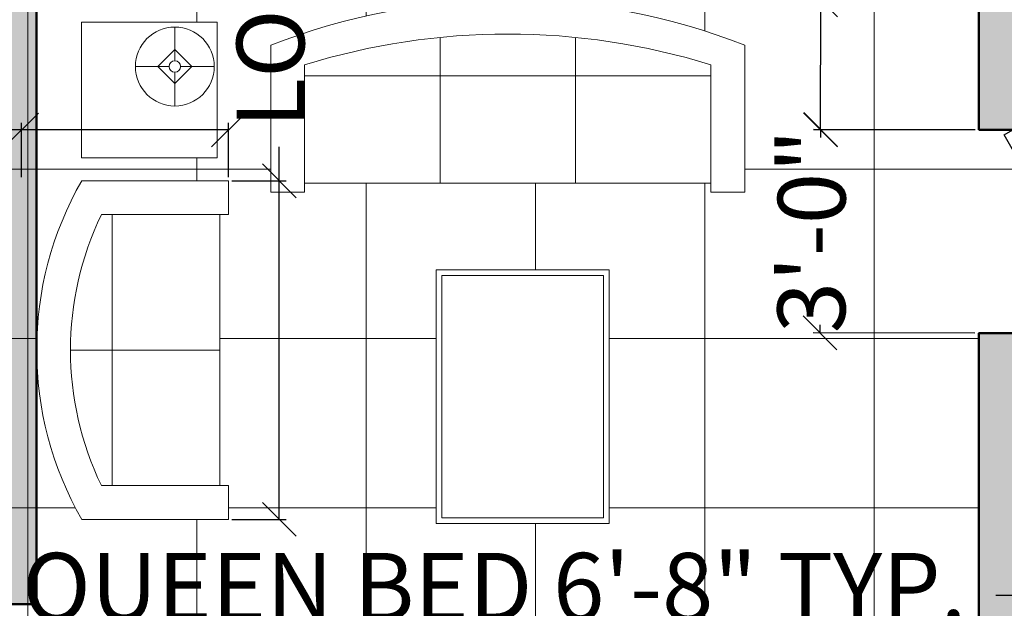
# Model space of a CAD drawing. Units: inches. Extents: x 2371 to 3019, y 129 to 700.
# Tile 8 of 14: x 2579 to 2753, y 432 to 537. Entities that reach past the tile are written whole.
import ezdxf

# ---------------------------------------------------------------- set-up
doc = ezdxf.new("R2010")
doc.units = ezdxf.units.IN
for name, color, linetype, lineweight in [('A-ANNO-DIMS', 2, 'Continuous', 18), ('A-DOOR', 4, 'Continuous', 25), ('A-FLOR-PATT', 252, 'Continuous', 13), ('A-FURN', 8, 'Continuous', 18), ('A-WALL', 7, 'Continuous', 50), ('A-WALL-PATT', 8, 'Continuous', 13)]:
    doc.layers.add(name, color=color, linetype=linetype, lineweight=lineweight)
doc.styles.get("Standard").update_dxf_attribs({"font": 'arial.ttf'})
doc.dimstyles.new('ISO-25', dxfattribs={"dimtxt": 12, "dimasz": 6, "dimexe": 1.25, "dimexo": 0.625, "dimtad": 0, "dimdec": 1, "dimlunit": 3, "dimtxsty": 'Standard', "dimblk": 'OBLIQUE', "dimblk1": 'ORIGIN2', "dimblk2": 'OBLIQUE', "dimcen": 2.5, "dimadec": 0, "dimazin": 0, "dimtfac": 1, "dimtdec": 1, "dimtmove": 0, "dimatfit": 3, "dimldrblk": 'OBLIQUE', "dimfxl": 1, "dimarcsym": 0})

# ---------------------------------------------------------------- blocks, each defined once
blk = doc.blocks.new('Sofa - Roundback Loveseat 5 ft.')
for p, q in [((0, -32.44198), (0, -5.99998)), ((-24, -33.99998), (-24, -11.46958)), ((24.00004, -33.99998), (24.00004, -11.46958)), ((-23.9998, -13.38178), (23.99986, -13.38178)), ((-24, -32.44198), (24.00004, -32.44198))]:
    blk.add_line(p, q)
for points in [[(-24, -33.99998), (-30, -33.99998), (-30, -7.99998)], [(30.00004, -7.99998), (30.00004, -33.99998), (24.00004, -33.99998)]]:
    blk.add_lwpolyline(points)
for centre, radius, start, end in [((0, -60.24998), 60.24998, 60.13715, 119.8628), ((0, -61.38438), 55.38444, 64.32083, 115.6792)]:
    blk.add_arc(centre, radius, start, end)
blk = doc.blocks.new('Sofa - Roundback 7 ft.')
for p, q in [((-12.00002, -32.4421), (-12.00003, -6.5971)), ((11.99997, -32.4421), (11.99998, -6.5971)), ((-36.000027, -34), (-36.000027, -11.4696)), ((35.99998, -34), (35.99998, -11.4696)), ((-35.999844, -13.3819), (35.9998, -13.3819)), ((-36.000027, -32.4421), (35.99998, -32.4421))]:
    blk.add_line(p, q)
for points in [[(-36.000027, -34), (-42.000027, -34), (-42.000027, -8)], [(41.99998, -8), (41.99998, -34), (35.99998, -34)]]:
    blk.add_lwpolyline(points)
for centre, radius, start, end in [((0, -114.25), 114.25, 68.43141, 111.5686), ((-0.00001, -127.1968), 121.1968, 72.72033, 107.2797)]:
    blk.add_arc(centre, radius, start, end)
blk = doc.blocks.new('Lamp - Table')
for p, q in [((0, 7), (0, 1)), ((0, 3), (-3, 0)), ((3, 0), (0, 3)), ((-1, 0), (-7, 0)), ((-3, 0), (0, -3)), ((0, -3), (3, 0)), ((1, 0), (7, 0)), ((0, -1), (0, -7))]:
    blk.add_line(p, q)
for radius in [7, 1]:
    blk.add_circle((0, 0), radius)
blk = doc.blocks.new('*U10')
for p, q in [((0, 0), (0, -6)), ((36, 0), (36, -6))]:
    blk.add_line(p, q)
blk.add_lwpolyline([(0, 0), (31.18, 18), (32.05, 16.48), (0.87, -1.52)], close=True)
blk.add_arc((0, 0), 36, 0, 30)
blk = doc.blocks.new('_Oblique')
at = {"color": 0, "linetype": 'ByBlock', "lineweight": -2}
blk.add_line((-0.5, -0.5), (0.5, 0.5), dxfattribs=at)
blk = doc.blocks.new('*D24')
at = {"layer": 'A-ANNO-DIMS', "color": 0, "lineweight": -2, "transparency": 16777216}
for p, q in [((2757.61, 423.1), (2757.61, 435.73)), ((2837.61, 423.1), (2837.61, 435.73)), ((2757.61, 434.48), (2751.61, 434.48)), ((2837.61, 434.48), (2757.61, 434.48))]:
    blk.add_line(p, q, dxfattribs=at)
at = {"layer": 'Defpoints', "color": 0, "lineweight": 25, "transparency": 16777216}
for p in [(2757.61, 434.48), (2757.61, 422.48), (2837.61, 422.48)]:
    blk.add_point(p, dxfattribs=at)
at = {"layer": 'A-ANNO-DIMS', "color": 0, "lineweight": -2, "transparency": 16777216, "xscale": 6, "yscale": 6, "zscale": 6, "rotation": 180}
blk.add_blockref('_Oblique', (2757.61, 434.48), dxfattribs=at)
at = {"layer": 'A-ANNO-DIMS', "color": 0, "lineweight": -2, "transparency": 16777216, "xscale": 6, "yscale": 6, "zscale": 6}
blk.add_blockref('_Oblique', (2837.61, 434.48), dxfattribs=at)
at = {"layer": 'A-ANNO-DIMS', "color": 0, "transparency": 16777216, "insert": (2662.72, 434.48), "char_height": 12, "attachment_point": 5}
blk.add_mtext('QUEEN BED 6\'-8" TYP.', dxfattribs=at)
blk = doc.blocks.new('_Origin2')
at = {"color": 0, "linetype": 'ByBlock', "lineweight": -2}
blk.add_line((-0.5, 0), (-1, 0), dxfattribs=at)
for radius in [0.5, 0.25]:
    blk.add_circle((0, 0), radius, dxfattribs=at)
blk = doc.blocks.new('*D32')
at = {"layer": 'A-ANNO-DIMS', "color": 0, "lineweight": -2, "transparency": 16777216}
for p, q in [((2624.61, 507.98), (2624.61, 513.98)), ((2616.23, 507.98), (2625.86, 507.98)), ((2624.61, 447.98), (2624.61, 507.98)), ((2616.23, 447.98), (2625.86, 447.98))]:
    blk.add_line(p, q, dxfattribs=at)
at = {"layer": 'Defpoints', "color": 0, "lineweight": 25, "transparency": 16777216}
for p in [(2615.61, 507.98), (2624.61, 507.98), (2615.61, 447.98)]:
    blk.add_point(p, dxfattribs=at)
at = {"layer": 'A-ANNO-DIMS', "color": 0, "lineweight": -2, "transparency": 16777216, "xscale": 6, "yscale": 6, "zscale": 6}
for p, rotation in [((2624.61, 507.98), 90), ((2624.61, 447.98), 270)]:
    blk.add_blockref('_Oblique', p, dxfattribs=dict(at, rotation=rotation))
at = {"layer": 'A-ANNO-DIMS', "color": 0, "transparency": 16777216, "insert": (2624.61, 576.87), "char_height": 12, "attachment_point": 5, "rotation": 90}
blk.add_mtext('LOVESEAT 5\'-0"', dxfattribs=at)
blk = doc.blocks.new('*D33')
at = {"layer": 'A-ANNO-DIMS', "color": 0, "lineweight": -2, "transparency": 16777216}
for p, q in [((2578.94, 516.98), (2572.94, 516.98)), ((2578.94, 508.6), (2578.94, 518.23)), ((2615.61, 516.98), (2578.94, 516.98)), ((2615.61, 508.6), (2615.61, 518.23))]:
    blk.add_line(p, q, dxfattribs=at)
at = {"layer": 'Defpoints', "color": 0, "lineweight": 25, "transparency": 16777216}
for p in [(2578.94, 516.98), (2578.94, 507.98), (2615.61, 507.98)]:
    blk.add_point(p, dxfattribs=at)
at = {"layer": 'A-ANNO-DIMS', "color": 0, "lineweight": -2, "transparency": 16777216, "xscale": 6, "yscale": 6, "zscale": 6, "rotation": 180}
blk.add_blockref('_Oblique', (2578.94, 516.98), dxfattribs=at)
at = {"layer": 'A-ANNO-DIMS', "color": 0, "lineweight": -2, "transparency": 16777216, "xscale": 6, "yscale": 6, "zscale": 6}
blk.add_blockref('_Oblique', (2615.61, 516.98), dxfattribs=at)
at = {"layer": 'A-ANNO-DIMS', "color": 0, "transparency": 16777216, "insert": (2542.39, 516.98), "char_height": 12, "attachment_point": 5}
blk.add_mtext('3\'-0 1/2"', dxfattribs=at)
blk = doc.blocks.new('*D72')
at = {"layer": 'A-ANNO-DIMS', "color": 0, "lineweight": -2, "transparency": 16777216}
for p, q in [((2747.96, 516.99), (2719.29, 517.05)), ((2720.54, 517.05), (2720.54, 515.62)), ((2720.46, 481.05), (2720.47, 482.48)), ((2747.89, 480.99), (2719.21, 481.05))]:
    blk.add_line(p, q, dxfattribs=at)
at = {"layer": 'Defpoints', "color": 0, "lineweight": 25, "transparency": 16777216}
for p in [(2720.54, 517.05), (2748.59, 516.99), (2748.51, 480.99)]:
    blk.add_point(p, dxfattribs=at)
at = {"layer": 'A-ANNO-DIMS', "color": 0, "lineweight": -2, "transparency": 16777216, "xscale": 6, "yscale": 6, "zscale": 6}
for p, rotation in [((2720.54, 517.05), 89.87829389996865), ((2720.46, 481.05), 269.8782938999687)]:
    blk.add_blockref('_Oblique', p, dxfattribs=dict(at, rotation=rotation))
at = {"layer": 'A-ANNO-DIMS', "color": 0, "transparency": 16777216, "insert": (2720.5, 499.05), "char_height": 12, "attachment_point": 5, "rotation": 89.8783}
blk.add_mtext('3\'-0"', dxfattribs=at)
blk = doc.blocks.new('*D73')
at = {"layer": 'A-ANNO-DIMS', "color": 0, "lineweight": -2, "transparency": 16777216}
for p, q in [((2720.56, 540), (2720.56, 546)), ((2747.98, 539.98), (2719.31, 540)), ((2720.54, 517.01), (2720.56, 540)), ((2747.96, 516.99), (2719.29, 517.01))]:
    blk.add_line(p, q, dxfattribs=at)
at = {"layer": 'Defpoints', "color": 0, "lineweight": 25, "transparency": 16777216}
for p in [(2720.56, 540), (2748.61, 539.98), (2748.59, 516.99)]:
    blk.add_point(p, dxfattribs=at)
at = {"layer": 'A-ANNO-DIMS', "color": 0, "lineweight": -2, "transparency": 16777216, "xscale": 6, "yscale": 6, "zscale": 6}
for p, rotation in [((2720.56, 540), 89.96084939784976), ((2720.54, 517.01), 269.9608493978498)]:
    blk.add_blockref('_Oblique', p, dxfattribs=dict(at, rotation=rotation))
at = {"layer": 'A-ANNO-DIMS', "color": 0, "transparency": 16777216, "insert": (2720.57, 566.67), "char_height": 12, "attachment_point": 5, "rotation": 89.9608}
blk.add_mtext('1\'-11"', dxfattribs=at)

msp = doc.modelspace()

# ---------------------------------------------------------------- hatches: boundary and pattern name
at = {"layer": 'A-FLOR-PATT'}
h = msp.add_hatch(dxfattribs=at)
h.set_pattern_fill('_USER', color=256, scale=30, pattern_type=0)
h.set_pattern_definition([(0, (0, 0), (0, 30), [])])
h.paths.add_polyline_path([(2913.11, 498.98), (2827.61, 498.98), (2827.61, 531.98), (2832.11, 531.98), (2832.11, 537.98), (2833.61, 537.98), (2833.61, 605.98), (2818.35, 605.98, -1), (2796.86, 605.98), (2781.61, 605.98), (2781.61, 603.98), (2781.61, 533.98), (2757.61, 533.98), (2757.61, 531.98), (2797.61, 531.98), (2797.61, 522.98), (2757.61, 522.98), (2757.61, 516.98), (2754.59, 516.98), (2772.52, 485.76), (2771.01, 484.89), (2770.98, 484.93, -0.097552), (2757.61, 481.1), (2757.61, 422.48), (2837.61, 422.48), (2837.61, 362.48), (2757.61, 362.48), (2757.61, 303.98), (2835.86, 303.98, -0.09439), (2793.86, 311.98), (2793.86, 337.98), (2799.86, 337.98), (2799.86, 336.42), (2871.86, 336.42), (2871.86, 337.98), (2877.86, 337.98), (2877.86, 311.98, -0.09439), (2835.86, 303.98), (2913.11, 303.98), (2913.11, 383.18), (2904.11, 383.18), (2904.11, 419.18), (2913.11, 419.18)])
h.paths.add_polyline_path([(2788.88, 332.88), (2788.88, 308.88), (2764.88, 308.88), (2764.88, 332.88)], flags=16)
h.paths.add_polyline_path([(2788.4, 325.04, -1), (2774.4, 325.04, -1)], flags=0)
h.paths.add_polyline_path([(2781.4, 328.04), (2784.4, 325.04), (2781.4, 322.04), (2778.4, 325.04)], flags=0)
h.paths.add_polyline_path([(2782.4, 325.04, -1), (2780.4, 325.04, -1)], flags=0)
h.paths.add_polyline_path([(2748.61, 480.99), (2754.51, 480.98, 0.119303), (2770.98, 484.93), (2753.07, 516.1), (2754.59, 516.98), (2748.61, 516.98), (2748.61, 539.98), (2712.61, 539.98), (2665.11, 539.98, -0.09439), (2707.11, 531.98), (2707.11, 505.98), (2701.11, 505.98), (2701.11, 507.53), (2629.11, 507.53), (2629.11, 505.98), (2623.11, 505.98), (2623.11, 531.98, -0.09439), (2665.11, 539.98), (2581.61, 539.98), (2581.61, 522.98), (2581.61, 477.98, -0.131044), (2589.61, 507.98), (2615.61, 507.98), (2615.61, 501.98), (2614.05, 501.98), (2614.05, 453.98), (2615.61, 453.98), (2615.61, 447.98), (2589.61, 447.98, -0.131044), (2581.61, 477.98), (2581.61, 432.98), (2572.61, 432.98, 0.119303), (2556.14, 428.99), (2574.12, 397.85), (2572.61, 396.98), (2578.61, 396.98), (2581.61, 396.98), (2581.61, 390.98), (2748.61, 390.98)])
h.paths.add_polyline_path([(2683.1, 447.25), (2652.43, 447.25), (2652.43, 492.22), (2683.1, 492.22)], flags=16)
h.paths.add_polyline_path([(2682.1, 448.25), (2653.43, 448.25), (2653.43, 491.22), (2682.1, 491.22)], flags=0)
h.paths.add_polyline_path([(2613.58, 512.06), (2589.58, 512.06), (2589.58, 536.06), (2613.58, 536.06)], flags=16)
h.paths.add_polyline_path([(2599.1, 528.22, -1), (2613.1, 528.22, -1)], flags=0)
h.paths.add_polyline_path([(2609.1, 528.22), (2606.1, 525.22), (2603.1, 528.22), (2606.1, 531.22)], flags=0)
h.paths.add_polyline_path([(2607.1, 528.22, -1), (2605.1, 528.22, -1)], flags=0)
h.paths.add_polyline_path([(2581.61, 522.98), (2581.61, 621.98), (2572.61, 621.98), (2572.61, 522.98), (2572.61, 500.98), (2565.85, 500.98), (2565.85, 500.15), (2564.82, 500.15), (2561.16, 500.19), (2561.16, 500.17), (2560.13, 500.3), (2560.22, 500.98), (2556.38, 500.98), (2556.43, 500.22), (2555.4, 500.14), (2555.34, 500.98), (2551.07, 500.98), (2551.07, 500.15), (2550.04, 500.15), (2547.64, 500.19), (2547.64, 500.15), (2546.61, 500.15), (2541.79, 500.22), (2540.72, 500.13), (2540.65, 500.98), (2533.37, 500.98), (2533.37, 500.15), (2532.34, 500.15), (2529.13, 500.21), (2529.12, 500.13), (2528.09, 500.22), (2528.16, 500.98), (2523.23, 500.98), (2523.23, 500.15), (2522.2, 500.15), (2519.8, 500.21), (2519.8, 500.15), (2518.77, 500.15), (2514.45, 500.26), (2514.44, 500.14), (2513.41, 500.22), (2513.47, 500.98), (2509.62, 500.98), (2509.71, 500.3), (2508.69, 500.17), (2508.58, 500.98), (2505.03, 500.98), (2505.03, 500.15), (2503.99, 500.15), (2501.07, 500.29), (2501.07, 500.15), (2500.04, 500.15), (2496.44, 500.37), (2496.44, 500.15), (2495.4, 500.15), (2492.55, 500.41), (2492.18, 500.35), (2492.09, 500.98), (2486.11, 500.98), (2486.11, 524.98), (2486.11, 531.98), (2490.61, 531.98), (2490.61, 537.98), (2492.11, 537.98), (2492.11, 605.98), (2476.85, 605.98, -1), (2455.36, 605.98), (2440.11, 605.98), (2440.11, 533.98), (2416.11, 533.98), (2416.11, 605.98), (2416.11, 621.98), (2536.61, 621.98), (2536.61, 630.98), (2407.11, 630.98), (2407.11, 363.98), (2416.11, 363.98), (2416.11, 431.48), (2496.11, 431.48), (2496.11, 371.48), (2416.11, 371.48), (2416.11, 303.98), (2494.36, 303.98, -0.09439), (2452.36, 311.98), (2452.36, 337.98), (2458.36, 337.98), (2458.36, 336.42), (2530.36, 336.42), (2530.36, 337.98), (2536.36, 337.98), (2536.36, 311.98, -0.09439), (2494.36, 303.98), (2572.61, 303.98), (2572.61, 381.98), (2572.61, 396.98), (2554.61, 428.15), (2556.12, 429.03), (2556.14, 428.99, -0.119303), (2572.61, 432.98), (2578.61, 432.98), (2581.61, 432.98)])
h.paths.add_polyline_path([(2450.11, 500.98), (2444.5, 500.98), (2444.44, 500.14), (2443.41, 500.22), (2443.47, 500.98), (2439.62, 500.98), (2439.71, 500.3), (2438.69, 500.17), (2438.58, 500.98), (2435.02, 500.98), (2435.02, 500.15), (2433.99, 500.15), (2433.99, 500.98), (2431.07, 500.98), (2431.07, 500.15), (2430.04, 500.15), (2430.04, 500.98), (2426.43, 500.98), (2426.43, 500.15), (2425.4, 500.15), (2425.4, 500.98), (2423.13, 500.98), (2423.2, 500.5), (2422.18, 500.35), (2422.09, 500.98), (2416.11, 500.98), (2416.11, 524.98), (2416.11, 531.98), (2450.11, 531.98), (2450.11, 522.98)], flags=16)
h.paths.add_polyline_path([(2449.11, 501.98), (2417.11, 501.98), (2417.11, 522.98), (2417.11, 523.98), (2449.11, 523.98)], flags=0)
h.paths.add_polyline_path([(2420.7, 510.73), (2419.36, 520.07), (2420.38, 520.22), (2421.74, 510.73), (2425.4, 510.73), (2425.4, 520.07), (2426.43, 520.07), (2426.43, 510.73), (2430.04, 510.73), (2430.04, 520.07), (2431.07, 520.07), (2431.07, 510.73), (2433.99, 510.73), (2433.99, 520.07), (2435.02, 520.07), (2435.02, 510.73), (2437.35, 510.73), (2436.18, 519.93), (2437.2, 520.06), (2438.39, 510.73), (2444.17, 510.73), (2444.85, 520.08), (2445.88, 520.01), (2445.21, 510.73)], flags=0)
h.paths.add_polyline_path([(2446.94, 336.11), (2446.94, 312.11), (2422.94, 312.11), (2422.94, 336.11)], flags=16)
h.paths.add_polyline_path([(2446.46, 328.27, -1), (2432.46, 328.27, -1)], flags=0)
h.paths.add_polyline_path([(2439.46, 331.27), (2442.46, 328.27), (2439.46, 325.27), (2436.46, 328.27)], flags=0)
h.paths.add_polyline_path([(2440.46, 328.27, -1), (2438.46, 328.27, -1)], flags=0)
h.paths.add_polyline_path([(2816, 444.88), (2866.87, 444.88), (2866.87, 463.54), (2816, 463.54)], flags=24)
h.paths.add_polyline_path([(2794.21, 558.3), (2833.34, 558.3), (2833.34, 576.96), (2794.21, 576.96)], flags=24)
h.paths.add_polyline_path([(2651.69, 411.53), (2711.04, 411.53), (2711.04, 430.19), (2651.69, 430.19)], flags=24)
h.paths.add_polyline_path([(2494.09, 444.88), (2544.97, 444.88), (2544.97, 463.54), (2494.09, 463.54)], flags=24)
h.paths.add_polyline_path([(2444.55, 565.02), (2483.69, 565.02), (2483.69, 583.68), (2444.55, 583.68)], flags=24)
h = msp.add_hatch(dxfattribs=at)
h.set_pattern_fill('_USER', color=256, scale=30, angle=90, pattern_type=0)
h.set_pattern_definition([(90, (0, 0), (-30, 2e-15), [])])
h.paths.add_polyline_path([(2913.11, 498.98), (2827.61, 498.98), (2827.61, 531.98), (2832.11, 531.98), (2832.11, 537.98), (2833.61, 537.98), (2833.61, 605.98), (2818.35, 605.98, -1), (2796.86, 605.98), (2781.61, 605.98), (2781.61, 603.98), (2781.61, 533.98), (2757.61, 533.98), (2757.61, 531.98), (2797.61, 531.98), (2797.61, 522.98), (2757.61, 522.98), (2757.61, 516.98), (2754.59, 516.98), (2772.52, 485.76), (2771.01, 484.89), (2770.98, 484.93, -0.097552), (2757.61, 481.1), (2757.61, 422.48), (2837.61, 422.48), (2837.61, 362.48), (2757.61, 362.48), (2757.61, 303.98), (2835.86, 303.98, -0.09439), (2793.86, 311.98), (2793.86, 337.98), (2799.86, 337.98), (2799.86, 336.42), (2871.86, 336.42), (2871.86, 337.98), (2877.86, 337.98), (2877.86, 311.98, -0.09439), (2835.86, 303.98), (2913.11, 303.98), (2913.11, 383.18), (2904.11, 383.18), (2904.11, 419.18), (2913.11, 419.18)])
h.paths.add_polyline_path([(2788.88, 332.88), (2788.88, 308.88), (2764.88, 308.88), (2764.88, 332.88)], flags=16)
h.paths.add_polyline_path([(2788.4, 325.04, -1), (2774.4, 325.04, -1)], flags=0)
h.paths.add_polyline_path([(2781.4, 328.04), (2784.4, 325.04), (2781.4, 322.04), (2778.4, 325.04)], flags=0)
h.paths.add_polyline_path([(2782.4, 325.04, -1), (2780.4, 325.04, -1)], flags=0)
h.paths.add_polyline_path([(2748.61, 480.99), (2754.51, 480.98, 0.119303), (2770.98, 484.93), (2753.07, 516.1), (2754.59, 516.98), (2748.61, 516.98), (2748.61, 539.98), (2712.61, 539.98), (2665.11, 539.98, -0.09439), (2707.11, 531.98), (2707.11, 505.98), (2701.11, 505.98), (2701.11, 507.53), (2629.11, 507.53), (2629.11, 505.98), (2623.11, 505.98), (2623.11, 531.98, -0.09439), (2665.11, 539.98), (2581.61, 539.98), (2581.61, 522.98), (2581.61, 477.98, -0.131044), (2589.61, 507.98), (2615.61, 507.98), (2615.61, 501.98), (2614.05, 501.98), (2614.05, 453.98), (2615.61, 453.98), (2615.61, 447.98), (2589.61, 447.98, -0.131044), (2581.61, 477.98), (2581.61, 432.98), (2572.61, 432.98, 0.119303), (2556.14, 428.99), (2574.12, 397.85), (2572.61, 396.98), (2578.61, 396.98), (2581.61, 396.98), (2581.61, 390.98), (2748.61, 390.98)])
h.paths.add_polyline_path([(2683.1, 447.25), (2652.43, 447.25), (2652.43, 492.22), (2683.1, 492.22)], flags=16)
h.paths.add_polyline_path([(2682.1, 448.25), (2653.43, 448.25), (2653.43, 491.22), (2682.1, 491.22)], flags=0)
h.paths.add_polyline_path([(2613.58, 512.06), (2589.58, 512.06), (2589.58, 536.06), (2613.58, 536.06)], flags=16)
h.paths.add_polyline_path([(2599.1, 528.22, -1), (2613.1, 528.22, -1)], flags=0)
h.paths.add_polyline_path([(2609.1, 528.22), (2606.1, 525.22), (2603.1, 528.22), (2606.1, 531.22)], flags=0)
h.paths.add_polyline_path([(2607.1, 528.22, -1), (2605.1, 528.22, -1)], flags=0)
h.paths.add_polyline_path([(2581.61, 522.98), (2581.61, 621.98), (2572.61, 621.98), (2572.61, 522.98), (2572.61, 500.98), (2565.85, 500.98), (2565.85, 500.15), (2564.82, 500.15), (2561.16, 500.19), (2561.16, 500.17), (2560.13, 500.3), (2560.22, 500.98), (2556.38, 500.98), (2556.43, 500.22), (2555.4, 500.14), (2555.34, 500.98), (2551.07, 500.98), (2551.07, 500.15), (2550.04, 500.15), (2547.64, 500.19), (2547.64, 500.15), (2546.61, 500.15), (2541.79, 500.22), (2540.72, 500.13), (2540.65, 500.98), (2533.37, 500.98), (2533.37, 500.15), (2532.34, 500.15), (2529.13, 500.21), (2529.12, 500.13), (2528.09, 500.22), (2528.16, 500.98), (2523.23, 500.98), (2523.23, 500.15), (2522.2, 500.15), (2519.8, 500.21), (2519.8, 500.15), (2518.77, 500.15), (2514.45, 500.26), (2514.44, 500.14), (2513.41, 500.22), (2513.47, 500.98), (2509.62, 500.98), (2509.71, 500.3), (2508.69, 500.17), (2508.58, 500.98), (2505.03, 500.98), (2505.03, 500.15), (2503.99, 500.15), (2501.07, 500.29), (2501.07, 500.15), (2500.04, 500.15), (2496.44, 500.37), (2496.44, 500.15), (2495.4, 500.15), (2492.55, 500.41), (2492.18, 500.35), (2492.09, 500.98), (2486.11, 500.98), (2486.11, 524.98), (2486.11, 531.98), (2490.61, 531.98), (2490.61, 537.98), (2492.11, 537.98), (2492.11, 605.98), (2476.85, 605.98, -1), (2455.36, 605.98), (2440.11, 605.98), (2440.11, 533.98), (2416.11, 533.98), (2416.11, 605.98), (2416.11, 621.98), (2536.61, 621.98), (2536.61, 630.98), (2407.11, 630.98), (2407.11, 363.98), (2416.11, 363.98), (2416.11, 431.48), (2496.11, 431.48), (2496.11, 371.48), (2416.11, 371.48), (2416.11, 303.98), (2494.36, 303.98, -0.09439), (2452.36, 311.98), (2452.36, 337.98), (2458.36, 337.98), (2458.36, 336.42), (2530.36, 336.42), (2530.36, 337.98), (2536.36, 337.98), (2536.36, 311.98, -0.09439), (2494.36, 303.98), (2572.61, 303.98), (2572.61, 381.98), (2572.61, 396.98), (2554.61, 428.15), (2556.12, 429.03), (2556.14, 428.99, -0.119303), (2572.61, 432.98), (2578.61, 432.98), (2581.61, 432.98)])
h.paths.add_polyline_path([(2450.11, 500.98), (2444.5, 500.98), (2444.44, 500.14), (2443.41, 500.22), (2443.47, 500.98), (2439.62, 500.98), (2439.71, 500.3), (2438.69, 500.17), (2438.58, 500.98), (2435.02, 500.98), (2435.02, 500.15), (2433.99, 500.15), (2433.99, 500.98), (2431.07, 500.98), (2431.07, 500.15), (2430.04, 500.15), (2430.04, 500.98), (2426.43, 500.98), (2426.43, 500.15), (2425.4, 500.15), (2425.4, 500.98), (2423.13, 500.98), (2423.2, 500.5), (2422.18, 500.35), (2422.09, 500.98), (2416.11, 500.98), (2416.11, 524.98), (2416.11, 531.98), (2450.11, 531.98), (2450.11, 522.98)], flags=16)
h.paths.add_polyline_path([(2449.11, 501.98), (2417.11, 501.98), (2417.11, 522.98), (2417.11, 523.98), (2449.11, 523.98)], flags=0)
h.paths.add_polyline_path([(2420.7, 510.73), (2419.36, 520.07), (2420.38, 520.22), (2421.74, 510.73), (2425.4, 510.73), (2425.4, 520.07), (2426.43, 520.07), (2426.43, 510.73), (2430.04, 510.73), (2430.04, 520.07), (2431.07, 520.07), (2431.07, 510.73), (2433.99, 510.73), (2433.99, 520.07), (2435.02, 520.07), (2435.02, 510.73), (2437.35, 510.73), (2436.18, 519.93), (2437.2, 520.06), (2438.39, 510.73), (2444.17, 510.73), (2444.85, 520.08), (2445.88, 520.01), (2445.21, 510.73)], flags=0)
h.paths.add_polyline_path([(2446.94, 336.11), (2446.94, 312.11), (2422.94, 312.11), (2422.94, 336.11)], flags=16)
h.paths.add_polyline_path([(2446.46, 328.27, -1), (2432.46, 328.27, -1)], flags=0)
h.paths.add_polyline_path([(2439.46, 331.27), (2442.46, 328.27), (2439.46, 325.27), (2436.46, 328.27)], flags=0)
h.paths.add_polyline_path([(2440.46, 328.27, -1), (2438.46, 328.27, -1)], flags=0)
h.paths.add_polyline_path([(2816, 444.88), (2866.87, 444.88), (2866.87, 463.54), (2816, 463.54)], flags=24)
h.paths.add_polyline_path([(2794.21, 558.3), (2833.34, 558.3), (2833.34, 576.96), (2794.21, 576.96)], flags=24)
h.paths.add_polyline_path([(2651.69, 411.53), (2711.04, 411.53), (2711.04, 430.19), (2651.69, 430.19)], flags=24)
h.paths.add_polyline_path([(2494.09, 444.88), (2544.97, 444.88), (2544.97, 463.54), (2494.09, 463.54)], flags=24)
h.paths.add_polyline_path([(2444.55, 565.02), (2483.69, 565.02), (2483.69, 583.68), (2444.55, 583.68)], flags=24)
at = {"layer": 'A-WALL-PATT'}
h = msp.add_hatch(color=256, dxfattribs=at)
h.dxf.hatch_style = 1
h.paths.add_polyline_path([(2536.61, 630.98), (2407.11, 630.98), (2407.11, 363.98), (2416.11, 363.98), (2416.11, 498.98), (2416.11, 522.98), (2416.11, 531.98), (2416.11, 603.98), (2416.11, 621.98), (2536.61, 621.98)])
h.paths.add_polyline_path([(2630.98, 630.98), (2560.61, 630.98), (2560.61, 621.98), (2630.98, 621.98)])
h.paths.add_polyline_path([(2878.11, 630.98), (2699.23, 630.98), (2699.23, 621.98), (2878.11, 621.98)])
h.paths.add_polyline_path([(2496.61, 621.98), (2492.11, 621.98), (2492.11, 569.98), (2496.61, 569.98)], flags=17)
h.paths.add_polyline_path([(2581.61, 621.98), (2572.61, 621.98), (2572.61, 522.98), (2572.61, 498.98), (2572.61, 432.98), (2578.61, 432.98), (2581.61, 432.98), (2581.61, 522.98)])
h.paths.add_polyline_path([(2572.61, 531.98), (2486.11, 531.98), (2486.11, 522.98), (2572.61, 522.98)])
h.paths.add_polyline_path([(2450.11, 531.98), (2440.11, 531.98), (2416.11, 531.98), (2416.11, 522.98), (2450.11, 522.98)], flags=17)
h.paths.add_polyline_path([(2416.11, 315.98), (2407.11, 315.98), (2407.11, 294.98), (2458.11, 294.98), (2458.11, 303.98), (2416.11, 303.98)])
h.paths.add_polyline_path([(2757.61, 303.98), (2530.61, 303.98), (2530.61, 294.98), (2757.61, 294.98)])
h.paths.add_polyline_path([(2581.61, 381.98), (2605.61, 381.98), (2617.61, 381.98), (2617.61, 390.98), (2581.61, 390.98), (2581.61, 396.98), (2572.61, 396.98), (2572.61, 381.98), (2572.61, 303.98), (2581.61, 303.98)])
h.paths.add_polyline_path([(2757.61, 480.98), (2748.61, 480.98), (2748.61, 381.98), (2748.61, 303.98), (2757.61, 303.98), (2757.61, 381.98), (2757.61, 422.48)])
h.paths.add_polyline_path([(2797.61, 531.98), (2757.61, 531.98), (2757.61, 603.98), (2757.61, 621.98), (2748.61, 621.98), (2748.61, 516.99), (2754.59, 516.98), (2757.61, 516.98), (2757.61, 522.98), (2797.61, 522.98)])
h.paths.add_polyline_path([(2913.11, 531.98), (2827.61, 531.98), (2827.61, 522.98), (2913.11, 522.98)])
h.paths.add_polyline_path([(2923.11, 630.98), (2902.11, 630.98), (2902.11, 621.98), (2914.11, 621.98), (2914.11, 363.98), (2923.11, 363.98)])
h.paths.add_polyline_path([(2923.11, 315.98), (2914.11, 315.98), (2914.11, 303.98), (2866.11, 303.98), (2866.11, 294.98), (2923.11, 294.98)])
h.paths.add_polyline_path([(2793.61, 303.98), (2757.61, 303.98), (2757.61, 294.98), (2793.61, 294.98)])

# ---------------------------------------------------------------- linework, layer by layer
at = {"layer": 'A-FURN'}
for points in [[(2589.58, 512.06), (2613.58, 512.06), (2613.58, 536.06), (2589.58, 536.06)], [(2652.43, 492.22), (2683.1, 492.22), (2683.1, 447.25), (2652.43, 447.25)], [(2653.43, 491.22), (2682.1, 491.22), (2682.1, 448.25), (2653.43, 448.25)]]:
    msp.add_lwpolyline(points, close=True, dxfattribs=at)
at = {"layer": 'A-WALL'}
for p, q in [((2581.61, 621.98), (2581.61, 522.98)), ((2748.61, 516.99), (2748.61, 621.98)), ((2581.61, 522.98), (2581.61, 432.98)), ((2757.61, 516.98), (2748.61, 516.98)), ((2748.61, 381.98), (2748.61, 480.98)), ((2757.61, 480.98), (2748.61, 480.98)), ((2572.61, 432.98), (2581.61, 432.98))]:
    msp.add_line(p, q, dxfattribs=at)

# ---------------------------------------------------------------- block references
at = {"layer": 'A-DOOR', "rotation": 269.8782938999684}
msp.add_blockref('*U10', (2754.59, 516.98), dxfattribs=at)
at = {"layer": 'A-FURN'}
for name, p in [('Sofa - Roundback 7 ft.', (2665.11, 539.98)), ('Lamp - Table', (2606.1, 528.22))]:
    msp.add_blockref(name, p, dxfattribs=at)
at = {"layer": 'A-FURN', "rotation": 90}
msp.add_blockref('Sofa - Roundback Loveseat 5 ft.', (2581.61, 477.98), dxfattribs=at)

# ---------------------------------------------------------------- dimensions: what is measured, and where the dimension line sits
at = {"layer": 'A-ANNO-DIMS'}
for base, p1, p2, angle, text, picture, middle in [((2624.61, 507.98), (2615.61, 447.98), (2615.61, 507.98), 90, 'LOVESEAT <>', '*D32', (2624.61, 576.87)), ((2757.61, 434.48), (2837.61, 422.48), (2757.61, 422.48), 180, 'QUEEN BED <> TYP.', '*D24', (2662.72, 434.48))]:
    dim = msp.add_linear_dim(base=base, p1=p1, p2=p2, angle=angle, text=text, dimstyle='ISO-25', override={"dimdec": 1, "dimrnd": 0, "dimzin": 1, "dimlunit": 4, "dimfrac": 2}, dxfattribs=at)
    dim.commit()
    dim.dimension.update_dxf_attribs({"geometry": picture, "text_midpoint": middle})
for base, p1, p2, angle, override, picture, middle in [((2720.56, 540), (2748.59, 516.99), (2748.61, 539.98), 89.9608, {"dimdec": 1, "dimlfac": 1, "dimrnd": 0, "dimzin": 1, "dimdsep": 46, "dimlunit": 4, "dimfrac": 2}, '*D73', (2720.57, 566.67)), ((2578.94, 516.98), (2615.61, 507.98), (2578.94, 507.98), 180, {"dimdec": 1, "dimrnd": 0, "dimzin": 1, "dimlunit": 4, "dimfrac": 2}, '*D33', (2542.39, 516.98)), ((2720.54, 517.05), (2748.51, 480.99), (2748.59, 516.99), 89.8783, {"dimdec": 1, "dimlfac": 1, "dimrnd": 0, "dimzin": 1, "dimdsep": 46, "dimlunit": 4, "dimfrac": 2}, '*D72', (2720.5, 499.05))]:
    dim = msp.add_linear_dim(base=base, p1=p1, p2=p2, angle=angle, dimstyle='ISO-25', override=override, dxfattribs=at)
    dim.commit()
    dim.dimension.update_dxf_attribs({"geometry": picture, "text_midpoint": middle})

doc.saveas('drawing.dxf')
